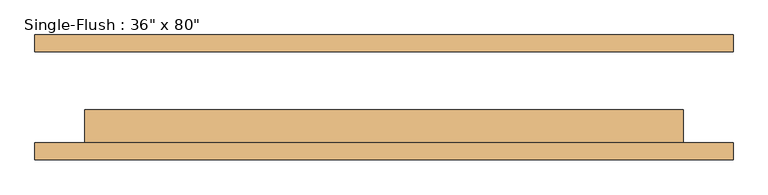
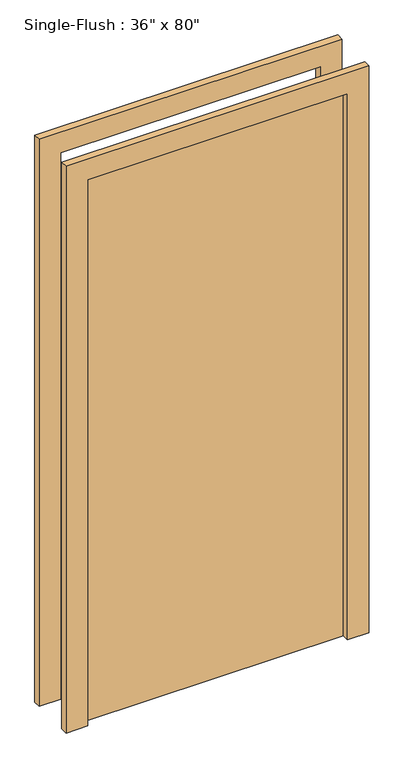
"""IFC4 building model written with IfcOpenShell, lengths in millimetres: door geometry."""

from ifc_helpers import new_model, si_unit, frame, origin, origin_with_axes, place, context, project, spatial, polyline, outline, extrude, source, transform, mapped, element, save


def door_798417c2(model_context):
    return source(origin(), model_context, "Body", "SweptSolid", [
        extrude(outline(polyline([(2108.2, -533.4), (0.0, -533.4), (0.0, -457.2), (2032.0, -457.2), (2032.0, 457.2), (0.0, 457.2), (0.0, 533.4), (2108.2, 533.4), (2108.2, -533.4)])), frame((0.0, -95.25, 0.0), z_axis=(0.0, 1.0, 0.0), x_axis=(0.0, 0.0, 1.0)), (0.0, 0.0, 1.0), 25.4),
        extrude(outline(polyline([(2108.2, 533.4), (2108.2, -533.4), (0.0, -533.4), (0.0, -457.2), (2032.0, -457.2), (2032.0, 457.2), (0.0, 457.2), (0.0, 533.4), (2108.2, 533.4)])), frame((0.0, 69.85, 0.0), z_axis=(0.0, 1.0, 0.0), x_axis=(0.0, 0.0, 1.0)), (0.0, 0.0, 1.0), 25.4),
        extrude(outline(polyline([(457.2, -19.05), (457.2, -69.85), (-457.2, -69.85), (-457.2, -19.05), (457.2, -19.05)])), origin_with_axes(), (0.0, 0.0, 1.0), 2032.0),
    ])


if __name__ == "__main__":
    model = new_model("IFC4")
    model_context = context("Model", 3, world=origin())
    ifc_project = project(units=[si_unit("LENGTHUNIT", "METRE", prefix="MILLI")], contexts=[model_context])
    site = spatial("IfcSite", under=ifc_project)
    building = spatial("IfcBuilding", under=site)
    placement = place(None, origin())
    door_shape = door_798417c2(model_context)
    element("IfcDoor", 1, ObjectType="Single-Flush : 36\" x 80\"", at=placement, inside=building, context=model_context, shape_type="MappedRepresentation", body=[
        mapped(door_shape, transform((0.0, 0.0, 0.0), x_axis=(1.0, 0.0, 0.0), y_axis=(0.0, 1.0, 0.0), z_axis=(0.0, 0.0, 1.0))),
    ])
    save(model, "model.ifc")

# Revit data of these elements
# Type "Single-Flush : 36\" x 80\""
#   Type Mark = "6"
#   Construction Type Id = "MDOOR"
#   Assembly Code = "C1020"
#   Analytic Construction = "Metal"
#   Thickness = 2"
#   Heat Transfer Coefficient (U) = 0.651978 BTU/(h·ft²·°F)
#   Height = 80"
#   Trim Projection Ext = 1"
#   Trim Projection Int = 1"
#   Trim Width = 3"
#   Width = 36"
#   Define Thermal Properties by = 1
#   Define Thermal Properties by = 1
#   Door Material = Door - Panel
#   Frame Material = Door - Frame
#   Visual Light Transmittance = 0
#   Solar Heat Gain Coefficient = 0
#   Function = (empty or 0)
#   Wall Closure = (empty or 0)
# Element 1 (IfcDoor, "Single-Flush : 36\" x 80\"")
#   Materials on its faces: "Door - Frame", "Door - Panel"
# Materials
#   "Door - Panel": class "Wood", colour RGB 210 159 95, transparency 0, Cost = 0
#   "Door - Frame": colour RGB 118 70 51, transparency 0, Cost = 0
